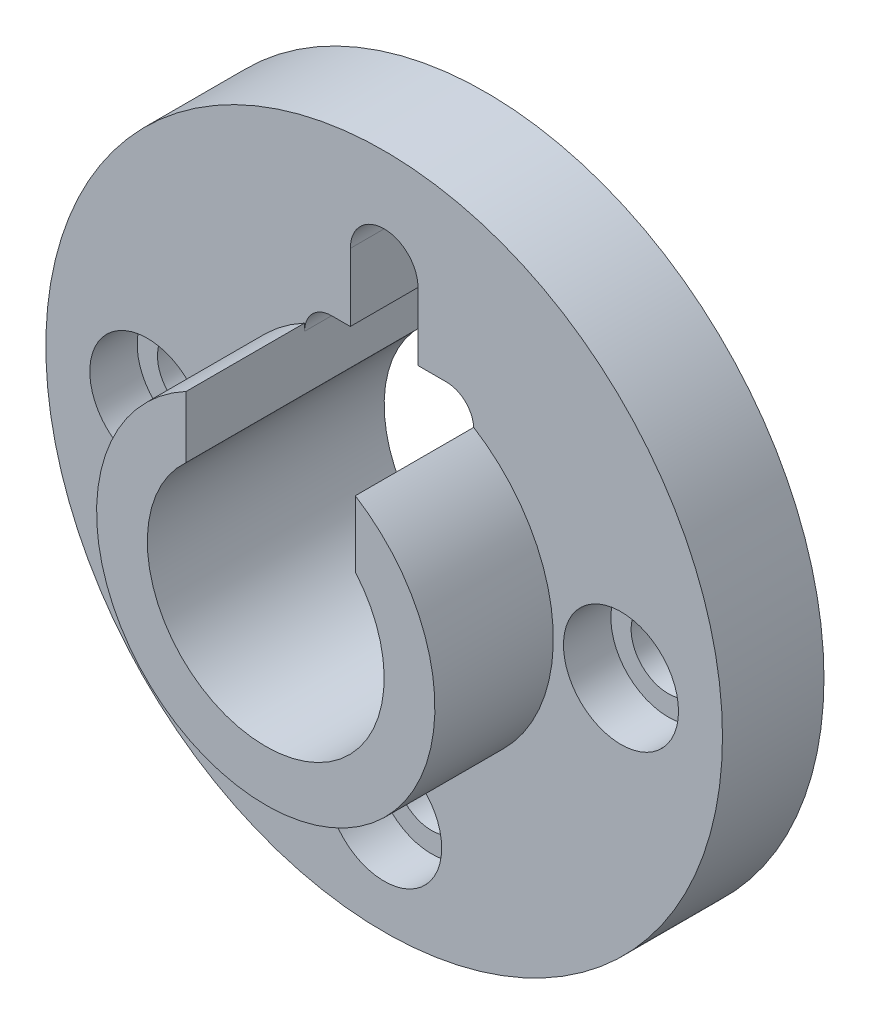
ISO-10303-21;
HEADER;
FILE_DESCRIPTION(('STEP AP214'),'2;1');
FILE_NAME('part.step','',(''),(''),'','','');
FILE_SCHEMA(('AUTOMOTIVE_DESIGN { 1 0 10303 214 1 1 1 1 }'));
ENDSEC;
DATA;
#1=APPLICATION_CONTEXT('core data for automotive mechanical design processes');
#2=APPLICATION_PROTOCOL_DEFINITION('international standard','automotive_design',2000,#1);
#3=PRODUCT_CONTEXT('',#1,'mechanical');
#4=PRODUCT('Part','Part','',(#3));
#5=PRODUCT_RELATED_PRODUCT_CATEGORY('part','',(#4));
#6=PRODUCT_DEFINITION_FORMATION('','',#4);
#7=PRODUCT_DEFINITION_CONTEXT('part definition',#1,'design');
#8=PRODUCT_DEFINITION('design','',#6,#7);
#9=PRODUCT_DEFINITION_SHAPE('','',#8);
#10=(LENGTH_UNIT() NAMED_UNIT(*) SI_UNIT(.MILLI.,.METRE.));
#11=(NAMED_UNIT(*) PLANE_ANGLE_UNIT() SI_UNIT($,.RADIAN.));
#12=(NAMED_UNIT(*) SI_UNIT($,.STERADIAN.) SOLID_ANGLE_UNIT());
#13=UNCERTAINTY_MEASURE_WITH_UNIT(LENGTH_MEASURE(1.E-05),#10,'distance_accuracy_value','');
#14=(GEOMETRIC_REPRESENTATION_CONTEXT(3) GLOBAL_UNCERTAINTY_ASSIGNED_CONTEXT((#13)) GLOBAL_UNIT_ASSIGNED_CONTEXT((#10,
#11,#12)) REPRESENTATION_CONTEXT('',''));
#15=CARTESIAN_POINT('',(0.,0.,0.));
#16=DIRECTION('',(0.,0.,1.));
#17=DIRECTION('',(1.,0.,0.));
#18=AXIS2_PLACEMENT_3D('',#15,#16,#17);
#19=CARTESIAN_POINT('',(-35.,0.,7.5));
#20=DIRECTION('',(0.,0.,-1.));
#21=DIRECTION('',(-1.,0.,0.));
#22=AXIS2_PLACEMENT_3D('',#19,#20,#21);
#23=CYLINDRICAL_SURFACE('',#22,5.5);
#24=CARTESIAN_POINT('',(-35.,0.,-7.5));
#25=DIRECTION('',(0.,0.,1.));
#26=DIRECTION('',(1.,0.,0.));
#27=AXIS2_PLACEMENT_3D('',#24,#25,#26);
#28=CIRCLE('',#27,5.5);
#29=CARTESIAN_POINT('',(-29.5,0.,-7.5));
#30=VERTEX_POINT('',#29);
#31=EDGE_CURVE('E245',#30,#30,#28,.T.);
#32=ORIENTED_EDGE('',*,*,#31,.F.);
#33=EDGE_LOOP('',(#32));
#34=FACE_BOUND('',#33,.T.);
#35=CARTESIAN_POINT('',(-35.,0.,0.5));
#36=DIRECTION('',(0.,0.,1.));
#37=DIRECTION('',(1.,0.,0.));
#38=AXIS2_PLACEMENT_3D('',#35,#36,#37);
#39=CIRCLE('',#38,5.5);
#40=CARTESIAN_POINT('',(-29.5,0.,0.5));
#41=VERTEX_POINT('',#40);
#42=EDGE_CURVE('E44',#41,#41,#39,.T.);
#43=ORIENTED_EDGE('',*,*,#42,.T.);
#44=EDGE_LOOP('',(#43));
#45=FACE_BOUND('',#44,.T.);
#46=ADVANCED_FACE('F41',(#34,#45),#23,.F.);
#47=CARTESIAN_POINT('',(35.,-2.44403693719019E-13,7.5));
#48=DIRECTION('',(0.,0.,-1.));
#49=DIRECTION('',(-1.,0.,0.));
#50=AXIS2_PLACEMENT_3D('',#47,#48,#49);
#51=CYLINDRICAL_SURFACE('',#50,5.5);
#52=CARTESIAN_POINT('',(35.,-2.44403693719019E-13,-7.5));
#53=DIRECTION('',(0.,0.,1.));
#54=DIRECTION('',(1.,0.,0.));
#55=AXIS2_PLACEMENT_3D('',#52,#53,#54);
#56=CIRCLE('',#55,5.5);
#57=CARTESIAN_POINT('',(40.5,-2.44403693719019E-13,-7.5));
#58=VERTEX_POINT('',#57);
#59=EDGE_CURVE('E242',#58,#58,#56,.T.);
#60=ORIENTED_EDGE('',*,*,#59,.F.);
#61=EDGE_LOOP('',(#60));
#62=FACE_BOUND('',#61,.T.);
#63=CARTESIAN_POINT('',(35.,-2.44403693719019E-13,0.5));
#64=DIRECTION('',(0.,0.,1.));
#65=DIRECTION('',(1.,0.,0.));
#66=AXIS2_PLACEMENT_3D('',#63,#64,#65);
#67=CIRCLE('',#66,5.5);
#68=CARTESIAN_POINT('',(40.5,-2.44403693719019E-13,0.5));
#69=VERTEX_POINT('',#68);
#70=EDGE_CURVE('E254',#69,#69,#67,.T.);
#71=ORIENTED_EDGE('',*,*,#70,.T.);
#72=EDGE_LOOP('',(#71));
#73=FACE_BOUND('',#72,.T.);
#74=ADVANCED_FACE('F351',(#62,#73),#51,.F.);
#75=CARTESIAN_POINT('',(-3.66605540578529E-13,-35.,7.5));
#76=DIRECTION('',(0.,0.,-1.));
#77=DIRECTION('',(-1.,0.,0.));
#78=AXIS2_PLACEMENT_3D('',#75,#76,#77);
#79=CYLINDRICAL_SURFACE('',#78,5.5);
#80=CARTESIAN_POINT('',(-3.66605540578529E-13,-35.,-7.5));
#81=DIRECTION('',(0.,0.,1.));
#82=DIRECTION('',(1.,0.,0.));
#83=AXIS2_PLACEMENT_3D('',#80,#81,#82);
#84=CIRCLE('',#83,5.5);
#85=CARTESIAN_POINT('',(5.49999999999963,-35.,-7.5));
#86=VERTEX_POINT('',#85);
#87=EDGE_CURVE('E239',#86,#86,#84,.T.);
#88=ORIENTED_EDGE('',*,*,#87,.F.);
#89=EDGE_LOOP('',(#88));
#90=FACE_BOUND('',#89,.T.);
#91=CARTESIAN_POINT('',(-3.66605540578529E-13,-35.,0.5));
#92=DIRECTION('',(0.,0.,1.));
#93=DIRECTION('',(1.,0.,0.));
#94=AXIS2_PLACEMENT_3D('',#91,#92,#93);
#95=CIRCLE('',#94,5.5);
#96=CARTESIAN_POINT('',(5.49999999999963,-35.,0.5));
#97=VERTEX_POINT('',#96);
#98=EDGE_CURVE('E251',#97,#97,#95,.T.);
#99=ORIENTED_EDGE('',*,*,#98,.T.);
#100=EDGE_LOOP('',(#99));
#101=FACE_BOUND('',#100,.T.);
#102=ADVANCED_FACE('F317',(#90,#101),#79,.F.);
#103=CARTESIAN_POINT('',(0.,0.,7.5));
#104=DIRECTION('',(0.,0.,1.));
#105=DIRECTION('',(1.,0.,0.));
#106=AXIS2_PLACEMENT_3D('',#103,#104,#105);
#107=PLANE('',#106);
#108=CARTESIAN_POINT('',(-35.,0.,7.5));
#109=DIRECTION('',(0.,0.,1.));
#110=DIRECTION('',(1.,0.,0.));
#111=AXIS2_PLACEMENT_3D('',#108,#109,#110);
#112=CIRCLE('',#111,8.5);
#113=CARTESIAN_POINT('',(-26.5,0.,7.5));
#114=VERTEX_POINT('',#113);
#115=EDGE_CURVE('E300',#114,#114,#112,.T.);
#116=ORIENTED_EDGE('',*,*,#115,.F.);
#117=EDGE_LOOP('',(#116));
#118=FACE_BOUND('',#117,.T.);
#119=CARTESIAN_POINT('',(35.,-2.44403693719019E-13,7.5));
#120=DIRECTION('',(0.,0.,1.));
#121=DIRECTION('',(1.,0.,0.));
#122=AXIS2_PLACEMENT_3D('',#119,#120,#121);
#123=CIRCLE('',#122,8.5);
#124=CARTESIAN_POINT('',(43.5,-2.44403693719019E-13,7.5));
#125=VERTEX_POINT('',#124);
#126=EDGE_CURVE('E297',#125,#125,#123,.T.);
#127=ORIENTED_EDGE('',*,*,#126,.F.);
#128=EDGE_LOOP('',(#127));
#129=FACE_BOUND('',#128,.T.);
#130=CARTESIAN_POINT('',(-3.66605540578529E-13,-35.,7.5));
#131=DIRECTION('',(0.,0.,1.));
#132=DIRECTION('',(1.,0.,0.));
#133=AXIS2_PLACEMENT_3D('',#130,#131,#132);
#134=CIRCLE('',#133,8.5);
#135=CARTESIAN_POINT('',(8.49999999999964,-35.,7.5));
#136=VERTEX_POINT('',#135);
#137=EDGE_CURVE('E292',#136,#136,#134,.T.);
#138=ORIENTED_EDGE('',*,*,#137,.F.);
#139=EDGE_LOOP('',(#138));
#140=FACE_BOUND('',#139,.T.);
#141=CARTESIAN_POINT('',(0.,0.,7.5));
#142=DIRECTION('',(0.,0.,1.));
#143=DIRECTION('',(1.,0.,0.));
#144=AXIS2_PLACEMENT_3D('',#141,#142,#143);
#145=CIRCLE('',#144,50.);
#146=CARTESIAN_POINT('',(50.,0.,7.5));
#147=VERTEX_POINT('',#146);
#148=EDGE_CURVE('E49',#147,#147,#145,.T.);
#149=ORIENTED_EDGE('',*,*,#148,.T.);
#150=EDGE_LOOP('',(#149));
#151=FACE_BOUND('',#150,.T.);
#152=CARTESIAN_POINT('',(9.23698245276787,21.,7.5));
#153=DIRECTION('',(0.,0.,1.));
#154=DIRECTION('',(-1.,0.,0.));
#155=AXIS2_PLACEMENT_3D('',#152,#153,#154);
#156=CIRCLE('',#155,4.);
#157=CARTESIAN_POINT('',(13.2369824527679,21.,7.5));
#158=VERTEX_POINT('',#157);
#159=CARTESIAN_POINT('',(9.23698245276784,25.,7.5));
#160=VERTEX_POINT('',#159);
#161=EDGE_CURVE('E194',#158,#160,#156,.T.);
#162=ORIENTED_EDGE('',*,*,#161,.F.);
#163=DIRECTION('',(0.,1.,0.));
#164=VECTOR('',#163,1.);
#165=CARTESIAN_POINT('',(13.2369824527679,0.,7.5));
#166=LINE('',#165,#164);
#167=CARTESIAN_POINT('',(13.2369824527679,21.2080714716147,7.5));
#168=VERTEX_POINT('',#167);
#169=EDGE_CURVE('E171',#158,#168,#166,.T.);
#170=ORIENTED_EDGE('',*,*,#169,.T.);
#171=CARTESIAN_POINT('',(0.,0.,7.5));
#172=DIRECTION('',(0.,0.,1.));
#173=DIRECTION('',(1.,0.,0.));
#174=AXIS2_PLACEMENT_3D('',#171,#172,#173);
#175=CIRCLE('',#174,25.);
#176=CARTESIAN_POINT('',(-11.7630175472321,22.059723891824,7.5));
#177=VERTEX_POINT('',#176);
#178=EDGE_CURVE('E170',#168,#177,#175,.F.);
#179=ORIENTED_EDGE('',*,*,#178,.T.);
#180=DIRECTION('',(0.,-1.,0.));
#181=VECTOR('',#180,1.);
#182=CARTESIAN_POINT('',(-11.7630175472321,0.,7.5));
#183=LINE('',#182,#181);
#184=CARTESIAN_POINT('',(-11.7630175472321,21.,7.5));
#185=VERTEX_POINT('',#184);
#186=EDGE_CURVE('E176',#177,#185,#183,.T.);
#187=ORIENTED_EDGE('',*,*,#186,.T.);
#188=CARTESIAN_POINT('',(-7.76301754723214,21.,7.5));
#189=DIRECTION('',(0.,0.,1.));
#190=DIRECTION('',(1.,0.,0.));
#191=AXIS2_PLACEMENT_3D('',#188,#189,#190);
#192=CIRCLE('',#191,4.);
#193=CARTESIAN_POINT('',(-7.76301754723211,25.,7.5));
#194=VERTEX_POINT('',#193);
#195=EDGE_CURVE('E190',#194,#185,#192,.T.);
#196=ORIENTED_EDGE('',*,*,#195,.F.);
#197=DIRECTION('',(-1.,0.,0.));
#198=VECTOR('',#197,1.);
#199=CARTESIAN_POINT('',(-7.76301754723211,25.,7.5));
#200=LINE('',#199,#198);
#201=CARTESIAN_POINT('',(-5.,25.,7.5));
#202=VERTEX_POINT('',#201);
#203=EDGE_CURVE('E189',#202,#194,#200,.T.);
#204=ORIENTED_EDGE('',*,*,#203,.F.);
#205=DIRECTION('',(0.,-1.,0.));
#206=VECTOR('',#205,1.);
#207=CARTESIAN_POINT('',(-5.,35.,7.5));
#208=LINE('',#207,#206);
#209=CARTESIAN_POINT('',(-5.,35.,7.5));
#210=VERTEX_POINT('',#209);
#211=EDGE_CURVE('E183',#210,#202,#208,.T.);
#212=ORIENTED_EDGE('',*,*,#211,.F.);
#213=CARTESIAN_POINT('',(0.,35.,7.5));
#214=DIRECTION('',(0.,0.,1.));
#215=DIRECTION('',(1.,0.,0.));
#216=AXIS2_PLACEMENT_3D('',#213,#214,#215);
#217=CIRCLE('',#216,5.);
#218=CARTESIAN_POINT('',(5.,35.,7.5));
#219=VERTEX_POINT('',#218);
#220=EDGE_CURVE('E181',#219,#210,#217,.T.);
#221=ORIENTED_EDGE('',*,*,#220,.F.);
#222=DIRECTION('',(0.,1.,0.));
#223=VECTOR('',#222,1.);
#224=CARTESIAN_POINT('',(5.,35.,7.5));
#225=LINE('',#224,#223);
#226=CARTESIAN_POINT('',(5.,25.,7.5));
#227=VERTEX_POINT('',#226);
#228=EDGE_CURVE('E196',#227,#219,#225,.T.);
#229=ORIENTED_EDGE('',*,*,#228,.F.);
#230=DIRECTION('',(-1.,0.,0.));
#231=VECTOR('',#230,1.);
#232=CARTESIAN_POINT('',(5.,25.,7.5));
#233=LINE('',#232,#231);
#234=EDGE_CURVE('E193',#160,#227,#233,.T.);
#235=ORIENTED_EDGE('',*,*,#234,.F.);
#236=EDGE_LOOP('',(#162,#170,#179,#187,#196,#204,#212,#221,#229,#235));
#237=FACE_BOUND('',#236,.T.);
#238=ADVANCED_FACE('F312',(#118,#129,#140,#151,#237),#107,.T.);
#239=CARTESIAN_POINT('',(0.,0.,-7.5));
#240=DIRECTION('',(0.,0.,1.));
#241=DIRECTION('',(1.,0.,0.));
#242=AXIS2_PLACEMENT_3D('',#239,#240,#241);
#243=PLANE('',#242);
#244=CARTESIAN_POINT('',(0.,0.,-7.5));
#245=DIRECTION('',(0.,0.,1.));
#246=DIRECTION('',(1.,0.,0.));
#247=AXIS2_PLACEMENT_3D('',#244,#245,#246);
#248=CIRCLE('',#247,50.);
#249=CARTESIAN_POINT('',(50.,0.,-7.5));
#250=VERTEX_POINT('',#249);
#251=EDGE_CURVE('E249',#250,#250,#248,.T.);
#252=ORIENTED_EDGE('',*,*,#251,.F.);
#253=EDGE_LOOP('',(#252));
#254=FACE_BOUND('',#253,.T.);
#255=ORIENTED_EDGE('',*,*,#31,.T.);
#256=EDGE_LOOP('',(#255));
#257=FACE_BOUND('',#256,.T.);
#258=ORIENTED_EDGE('',*,*,#59,.T.);
#259=EDGE_LOOP('',(#258));
#260=FACE_BOUND('',#259,.T.);
#261=ORIENTED_EDGE('',*,*,#87,.T.);
#262=EDGE_LOOP('',(#261));
#263=FACE_BOUND('',#262,.T.);
#264=DIRECTION('',(0.,1.,0.));
#265=VECTOR('',#264,1.);
#266=CARTESIAN_POINT('',(13.2369824527679,0.,-7.5));
#267=LINE('',#266,#265);
#268=CARTESIAN_POINT('',(13.2369824527679,21.,-7.5));
#269=VERTEX_POINT('',#268);
#270=CARTESIAN_POINT('',(13.2369824527679,21.2080714716147,-7.5));
#271=VERTEX_POINT('',#270);
#272=EDGE_CURVE('E169',#269,#271,#267,.T.);
#273=ORIENTED_EDGE('',*,*,#272,.F.);
#274=CARTESIAN_POINT('',(9.23698245276787,21.,-7.5));
#275=DIRECTION('',(0.,0.,1.));
#276=DIRECTION('',(-1.,0.,0.));
#277=AXIS2_PLACEMENT_3D('',#274,#275,#276);
#278=CIRCLE('',#277,4.);
#279=CARTESIAN_POINT('',(9.23698245276784,25.,-7.5));
#280=VERTEX_POINT('',#279);
#281=EDGE_CURVE('E211',#269,#280,#278,.T.);
#282=ORIENTED_EDGE('',*,*,#281,.T.);
#283=DIRECTION('',(-1.,0.,0.));
#284=VECTOR('',#283,1.);
#285=CARTESIAN_POINT('',(5.,25.,-7.5));
#286=LINE('',#285,#284);
#287=CARTESIAN_POINT('',(5.,25.,-7.5));
#288=VERTEX_POINT('',#287);
#289=EDGE_CURVE('E212',#280,#288,#286,.T.);
#290=ORIENTED_EDGE('',*,*,#289,.T.);
#291=DIRECTION('',(0.,1.,0.));
#292=VECTOR('',#291,1.);
#293=CARTESIAN_POINT('',(5.,35.,-7.5));
#294=LINE('',#293,#292);
#295=CARTESIAN_POINT('',(5.,35.,-7.5));
#296=VERTEX_POINT('',#295);
#297=EDGE_CURVE('E186',#288,#296,#294,.T.);
#298=ORIENTED_EDGE('',*,*,#297,.T.);
#299=CARTESIAN_POINT('',(0.,35.,-7.5));
#300=DIRECTION('',(0.,0.,1.));
#301=DIRECTION('',(1.,0.,0.));
#302=AXIS2_PLACEMENT_3D('',#299,#300,#301);
#303=CIRCLE('',#302,5.);
#304=CARTESIAN_POINT('',(-5.,35.,-7.5));
#305=VERTEX_POINT('',#304);
#306=EDGE_CURVE('E185',#296,#305,#303,.T.);
#307=ORIENTED_EDGE('',*,*,#306,.T.);
#308=DIRECTION('',(0.,-1.,0.));
#309=VECTOR('',#308,1.);
#310=CARTESIAN_POINT('',(-5.,35.,-7.5));
#311=LINE('',#310,#309);
#312=CARTESIAN_POINT('',(-5.,25.,-7.5));
#313=VERTEX_POINT('',#312);
#314=EDGE_CURVE('E201',#305,#313,#311,.T.);
#315=ORIENTED_EDGE('',*,*,#314,.T.);
#316=DIRECTION('',(-1.,0.,0.));
#317=VECTOR('',#316,1.);
#318=CARTESIAN_POINT('',(-7.76301754723211,25.,-7.5));
#319=LINE('',#318,#317);
#320=CARTESIAN_POINT('',(-7.76301754723211,25.,-7.5));
#321=VERTEX_POINT('',#320);
#322=EDGE_CURVE('E206',#313,#321,#319,.T.);
#323=ORIENTED_EDGE('',*,*,#322,.T.);
#324=CARTESIAN_POINT('',(-7.76301754723214,21.,-7.5));
#325=DIRECTION('',(0.,0.,1.));
#326=DIRECTION('',(1.,0.,0.));
#327=AXIS2_PLACEMENT_3D('',#324,#325,#326);
#328=CIRCLE('',#327,4.);
#329=CARTESIAN_POINT('',(-11.7630175472321,21.,-7.5));
#330=VERTEX_POINT('',#329);
#331=EDGE_CURVE('E207',#321,#330,#328,.T.);
#332=ORIENTED_EDGE('',*,*,#331,.T.);
#333=DIRECTION('',(0.,-1.,0.));
#334=VECTOR('',#333,1.);
#335=CARTESIAN_POINT('',(-11.7630175472321,0.,-7.5));
#336=LINE('',#335,#334);
#337=CARTESIAN_POINT('',(-11.7630175472321,22.059723891824,-7.5));
#338=VERTEX_POINT('',#337);
#339=EDGE_CURVE('E61',#338,#330,#336,.T.);
#340=ORIENTED_EDGE('',*,*,#339,.F.);
#341=CARTESIAN_POINT('',(0.,0.,-7.5));
#342=DIRECTION('',(0.,0.,1.));
#343=DIRECTION('',(1.,0.,0.));
#344=AXIS2_PLACEMENT_3D('',#341,#342,#343);
#345=CIRCLE('',#344,25.);
#346=EDGE_CURVE('E11',#271,#338,#345,.F.);
#347=ORIENTED_EDGE('',*,*,#346,.F.);
#348=EDGE_LOOP('',(#273,#282,#290,#298,#307,#315,#323,#332,#340,#347));
#349=FACE_BOUND('',#348,.T.);
#350=ADVANCED_FACE('F318',(#254,#257,#260,#263,#349),#243,.F.);
#351=CARTESIAN_POINT('',(0.,0.,7.5));
#352=DIRECTION('',(0.,0.,-1.));
#353=DIRECTION('',(-1.,0.,0.));
#354=AXIS2_PLACEMENT_3D('',#351,#352,#353);
#355=CYLINDRICAL_SURFACE('',#354,50.);
#356=ORIENTED_EDGE('',*,*,#148,.F.);
#357=EDGE_LOOP('',(#356));
#358=FACE_BOUND('',#357,.T.);
#359=ORIENTED_EDGE('',*,*,#251,.T.);
#360=EDGE_LOOP('',(#359));
#361=FACE_BOUND('',#360,.T.);
#362=ADVANCED_FACE('F43',(#358,#361),#355,.T.);
#363=CARTESIAN_POINT('',(0.,35.,7.5));
#364=DIRECTION('',(0.,0.,-1.));
#365=DIRECTION('',(-1.,0.,0.));
#366=AXIS2_PLACEMENT_3D('',#363,#364,#365);
#367=CYLINDRICAL_SURFACE('',#366,5.);
#368=ORIENTED_EDGE('',*,*,#306,.F.);
#369=DIRECTION('',(0.,0.,-1.));
#370=VECTOR('',#369,1.);
#371=CARTESIAN_POINT('',(5.,35.,7.5));
#372=LINE('',#371,#370);
#373=EDGE_CURVE('E199',#219,#296,#372,.T.);
#374=ORIENTED_EDGE('',*,*,#373,.F.);
#375=ORIENTED_EDGE('',*,*,#220,.T.);
#376=DIRECTION('',(0.,0.,-1.));
#377=VECTOR('',#376,1.);
#378=CARTESIAN_POINT('',(-5.,35.,7.5));
#379=LINE('',#378,#377);
#380=EDGE_CURVE('E237',#210,#305,#379,.T.);
#381=ORIENTED_EDGE('',*,*,#380,.T.);
#382=EDGE_LOOP('',(#368,#374,#375,#381));
#383=FACE_BOUND('',#382,.T.);
#384=ADVANCED_FACE('F347',(#383),#367,.F.);
#385=CARTESIAN_POINT('',(-5.,35.,7.5));
#386=DIRECTION('',(1.,0.,0.));
#387=DIRECTION('',(0.,1.,0.));
#388=AXIS2_PLACEMENT_3D('',#385,#386,#387);
#389=PLANE('',#388);
#390=ORIENTED_EDGE('',*,*,#314,.F.);
#391=ORIENTED_EDGE('',*,*,#380,.F.);
#392=ORIENTED_EDGE('',*,*,#211,.T.);
#393=DIRECTION('',(0.,0.,-1.));
#394=VECTOR('',#393,1.);
#395=CARTESIAN_POINT('',(-5.,25.,7.5));
#396=LINE('',#395,#394);
#397=EDGE_CURVE('E231',#202,#313,#396,.T.);
#398=ORIENTED_EDGE('',*,*,#397,.T.);
#399=EDGE_LOOP('',(#390,#391,#392,#398));
#400=FACE_BOUND('',#399,.T.);
#401=ADVANCED_FACE('F370',(#400),#389,.T.);
#402=CARTESIAN_POINT('',(-7.76301754723211,25.,7.5));
#403=DIRECTION('',(0.,-1.,0.));
#404=DIRECTION('',(0.,0.,-1.));
#405=AXIS2_PLACEMENT_3D('',#402,#403,#404);
#406=PLANE('',#405);
#407=ORIENTED_EDGE('',*,*,#322,.F.);
#408=ORIENTED_EDGE('',*,*,#397,.F.);
#409=ORIENTED_EDGE('',*,*,#203,.T.);
#410=DIRECTION('',(0.,0.,-1.));
#411=VECTOR('',#410,1.);
#412=CARTESIAN_POINT('',(-7.76301754723211,25.,7.5));
#413=LINE('',#412,#411);
#414=EDGE_CURVE('E235',#194,#321,#413,.T.);
#415=ORIENTED_EDGE('',*,*,#414,.T.);
#416=EDGE_LOOP('',(#407,#408,#409,#415));
#417=FACE_BOUND('',#416,.T.);
#418=ADVANCED_FACE('F371',(#417),#406,.T.);
#419=CARTESIAN_POINT('',(-7.76301754723214,21.,7.5));
#420=DIRECTION('',(0.,0.,-1.));
#421=DIRECTION('',(-1.,0.,0.));
#422=AXIS2_PLACEMENT_3D('',#419,#420,#421);
#423=CYLINDRICAL_SURFACE('',#422,4.);
#424=ORIENTED_EDGE('',*,*,#331,.F.);
#425=ORIENTED_EDGE('',*,*,#414,.F.);
#426=ORIENTED_EDGE('',*,*,#195,.T.);
#427=DIRECTION('',(0.,0.,-1.));
#428=VECTOR('',#427,1.);
#429=CARTESIAN_POINT('',(-11.7630175472321,21.,7.5));
#430=LINE('',#429,#428);
#431=EDGE_CURVE('E230',#185,#330,#430,.T.);
#432=ORIENTED_EDGE('',*,*,#431,.T.);
#433=EDGE_LOOP('',(#424,#425,#426,#432));
#434=FACE_BOUND('',#433,.T.);
#435=ADVANCED_FACE('F374',(#434),#423,.F.);
#436=CARTESIAN_POINT('',(-11.7630175472321,12.9569061964463,7.5));
#437=DIRECTION('',(1.,0.,0.));
#438=DIRECTION('',(0.,0.,-1.));
#439=AXIS2_PLACEMENT_3D('',#436,#437,#438);
#440=PLANE('',#439);
#441=DIRECTION('',(0.,0.,-1.));
#442=VECTOR('',#441,1.);
#443=CARTESIAN_POINT('',(-11.7630175472321,12.9569061964463,7.5));
#444=LINE('',#443,#442);
#445=CARTESIAN_POINT('',(-11.7630175472321,12.9569061964463,25.));
#446=VERTEX_POINT('',#445);
#447=CARTESIAN_POINT('',(-11.7630175472321,12.9569061964463,-10.));
#448=VERTEX_POINT('',#447);
#449=EDGE_CURVE('E229',#446,#448,#444,.T.);
#450=ORIENTED_EDGE('',*,*,#449,.T.);
#451=DIRECTION('',(0.,1.,0.));
#452=VECTOR('',#451,1.);
#453=CARTESIAN_POINT('',(-11.7630175472321,12.9569061964463,-10.));
#454=LINE('',#453,#452);
#455=CARTESIAN_POINT('',(-11.7630175472321,22.059723891824,-10.));
#456=VERTEX_POINT('',#455);
#457=EDGE_CURVE('E162',#448,#456,#454,.T.);
#458=ORIENTED_EDGE('',*,*,#457,.T.);
#459=DIRECTION('',(0.,0.,-1.));
#460=VECTOR('',#459,1.);
#461=CARTESIAN_POINT('',(-11.7630175472321,22.059723891824,25.));
#462=LINE('',#461,#460);
#463=EDGE_CURVE('E281',#338,#456,#462,.T.);
#464=ORIENTED_EDGE('',*,*,#463,.F.);
#465=ORIENTED_EDGE('',*,*,#339,.T.);
#466=ORIENTED_EDGE('',*,*,#431,.F.);
#467=ORIENTED_EDGE('',*,*,#186,.F.);
#468=CARTESIAN_POINT('',(-11.7630175472321,22.059723891824,25.));
#469=VERTEX_POINT('',#468);
#470=EDGE_CURVE('E174',#469,#177,#462,.T.);
#471=ORIENTED_EDGE('',*,*,#470,.F.);
#472=DIRECTION('',(0.,1.,0.));
#473=VECTOR('',#472,1.);
#474=CARTESIAN_POINT('',(-11.7630175472321,12.9569061964463,25.));
#475=LINE('',#474,#473);
#476=EDGE_CURVE('E157',#446,#469,#475,.T.);
#477=ORIENTED_EDGE('',*,*,#476,.F.);
#478=EDGE_LOOP('',(#450,#458,#464,#465,#466,#467,#471,#477));
#479=FACE_BOUND('',#478,.T.);
#480=ADVANCED_FACE('F278',(#479),#440,.T.);
#481=CARTESIAN_POINT('',(0.,0.,7.5));
#482=DIRECTION('',(0.,0.,-1.));
#483=DIRECTION('',(-1.,0.,0.));
#484=AXIS2_PLACEMENT_3D('',#481,#482,#483);
#485=CYLINDRICAL_SURFACE('',#484,17.5);
#486=DIRECTION('',(0.,0.,-1.));
#487=VECTOR('',#486,1.);
#488=CARTESIAN_POINT('',(13.2369824527679,11.4469338927556,7.5));
#489=LINE('',#488,#487);
#490=CARTESIAN_POINT('',(13.2369824527679,11.4469338927555,25.));
#491=VERTEX_POINT('',#490);
#492=CARTESIAN_POINT('',(13.2369824527679,11.4469338927555,-10.));
#493=VERTEX_POINT('',#492);
#494=EDGE_CURVE('E149',#491,#493,#489,.T.);
#495=ORIENTED_EDGE('',*,*,#494,.T.);
#496=CARTESIAN_POINT('',(0.,0.,-10.));
#497=DIRECTION('',(0.,0.,-1.));
#498=DIRECTION('',(1.,0.,0.));
#499=AXIS2_PLACEMENT_3D('',#496,#497,#498);
#500=CIRCLE('',#499,17.5);
#501=EDGE_CURVE('E269',#493,#448,#500,.T.);
#502=ORIENTED_EDGE('',*,*,#501,.T.);
#503=ORIENTED_EDGE('',*,*,#449,.F.);
#504=CARTESIAN_POINT('',(0.,0.,25.));
#505=DIRECTION('',(0.,0.,-1.));
#506=DIRECTION('',(1.,0.,0.));
#507=AXIS2_PLACEMENT_3D('',#504,#505,#506);
#508=CIRCLE('',#507,17.5);
#509=EDGE_CURVE('E153',#491,#446,#508,.T.);
#510=ORIENTED_EDGE('',*,*,#509,.F.);
#511=EDGE_LOOP('',(#495,#502,#503,#510));
#512=FACE_BOUND('',#511,.T.);
#513=ADVANCED_FACE('F381',(#512),#485,.F.);
#514=CARTESIAN_POINT('',(13.2369824527679,11.4469338927556,7.5));
#515=DIRECTION('',(-1.,0.,0.));
#516=DIRECTION('',(0.,0.,1.));
#517=AXIS2_PLACEMENT_3D('',#514,#515,#516);
#518=PLANE('',#517);
#519=DIRECTION('',(0.,0.,-1.));
#520=VECTOR('',#519,1.);
#521=CARTESIAN_POINT('',(13.2369824527679,21.,7.5));
#522=LINE('',#521,#520);
#523=EDGE_CURVE('E223',#158,#269,#522,.T.);
#524=ORIENTED_EDGE('',*,*,#523,.T.);
#525=ORIENTED_EDGE('',*,*,#272,.T.);
#526=DIRECTION('',(0.,0.,-1.));
#527=VECTOR('',#526,1.);
#528=CARTESIAN_POINT('',(13.2369824527679,21.2080714716147,25.));
#529=LINE('',#528,#527);
#530=CARTESIAN_POINT('',(13.2369824527679,21.2080714716147,-10.));
#531=VERTEX_POINT('',#530);
#532=EDGE_CURVE('E166',#271,#531,#529,.T.);
#533=ORIENTED_EDGE('',*,*,#532,.T.);
#534=DIRECTION('',(0.,-1.,0.));
#535=VECTOR('',#534,1.);
#536=CARTESIAN_POINT('',(13.2369824527679,11.4469338927556,-10.));
#537=LINE('',#536,#535);
#538=EDGE_CURVE('E264',#531,#493,#537,.T.);
#539=ORIENTED_EDGE('',*,*,#538,.T.);
#540=ORIENTED_EDGE('',*,*,#494,.F.);
#541=DIRECTION('',(0.,-1.,0.));
#542=VECTOR('',#541,1.);
#543=CARTESIAN_POINT('',(13.2369824527679,11.4469338927556,25.));
#544=LINE('',#543,#542);
#545=CARTESIAN_POINT('',(13.2369824527679,21.2080714716147,25.));
#546=VERTEX_POINT('',#545);
#547=EDGE_CURVE('E143',#546,#491,#544,.T.);
#548=ORIENTED_EDGE('',*,*,#547,.F.);
#549=EDGE_CURVE('E148',#546,#168,#529,.T.);
#550=ORIENTED_EDGE('',*,*,#549,.T.);
#551=ORIENTED_EDGE('',*,*,#169,.F.);
#552=EDGE_LOOP('',(#524,#525,#533,#539,#540,#548,#550,#551));
#553=FACE_BOUND('',#552,.T.);
#554=ADVANCED_FACE('F145',(#553),#518,.T.);
#555=CARTESIAN_POINT('',(9.23698245276787,21.,7.5));
#556=DIRECTION('',(0.,0.,-1.));
#557=DIRECTION('',(-1.,0.,0.));
#558=AXIS2_PLACEMENT_3D('',#555,#556,#557);
#559=CYLINDRICAL_SURFACE('',#558,4.);
#560=ORIENTED_EDGE('',*,*,#281,.F.);
#561=ORIENTED_EDGE('',*,*,#523,.F.);
#562=ORIENTED_EDGE('',*,*,#161,.T.);
#563=DIRECTION('',(0.,0.,-1.));
#564=VECTOR('',#563,1.);
#565=CARTESIAN_POINT('',(9.23698245276784,25.,7.5));
#566=LINE('',#565,#564);
#567=EDGE_CURVE('E224',#160,#280,#566,.T.);
#568=ORIENTED_EDGE('',*,*,#567,.T.);
#569=EDGE_LOOP('',(#560,#561,#562,#568));
#570=FACE_BOUND('',#569,.T.);
#571=ADVANCED_FACE('F331',(#570),#559,.F.);
#572=CARTESIAN_POINT('',(5.,25.,7.5));
#573=DIRECTION('',(0.,-1.,0.));
#574=DIRECTION('',(0.,0.,-1.));
#575=AXIS2_PLACEMENT_3D('',#572,#573,#574);
#576=PLANE('',#575);
#577=ORIENTED_EDGE('',*,*,#289,.F.);
#578=ORIENTED_EDGE('',*,*,#567,.F.);
#579=ORIENTED_EDGE('',*,*,#234,.T.);
#580=DIRECTION('',(0.,0.,-1.));
#581=VECTOR('',#580,1.);
#582=CARTESIAN_POINT('',(5.,25.,7.5));
#583=LINE('',#582,#581);
#584=EDGE_CURVE('E222',#227,#288,#583,.T.);
#585=ORIENTED_EDGE('',*,*,#584,.T.);
#586=EDGE_LOOP('',(#577,#578,#579,#585));
#587=FACE_BOUND('',#586,.T.);
#588=ADVANCED_FACE('F337',(#587),#576,.T.);
#589=CARTESIAN_POINT('',(5.,35.,7.5));
#590=DIRECTION('',(-1.,0.,0.));
#591=DIRECTION('',(0.,-1.,0.));
#592=AXIS2_PLACEMENT_3D('',#589,#590,#591);
#593=PLANE('',#592);
#594=ORIENTED_EDGE('',*,*,#297,.F.);
#595=ORIENTED_EDGE('',*,*,#584,.F.);
#596=ORIENTED_EDGE('',*,*,#228,.T.);
#597=ORIENTED_EDGE('',*,*,#373,.T.);
#598=EDGE_LOOP('',(#594,#595,#596,#597));
#599=FACE_BOUND('',#598,.T.);
#600=ADVANCED_FACE('F391',(#599),#593,.T.);
#601=CARTESIAN_POINT('',(0.,0.,-10.));
#602=DIRECTION('',(0.,0.,1.));
#603=DIRECTION('',(1.,0.,0.));
#604=AXIS2_PLACEMENT_3D('',#601,#602,#603);
#605=PLANE('',#604);
#606=CARTESIAN_POINT('',(0.,0.,-10.));
#607=DIRECTION('',(0.,0.,1.));
#608=DIRECTION('',(1.,0.,0.));
#609=AXIS2_PLACEMENT_3D('',#606,#607,#608);
#610=CIRCLE('',#609,25.);
#611=EDGE_CURVE('E261',#456,#531,#610,.T.);
#612=ORIENTED_EDGE('',*,*,#611,.F.);
#613=ORIENTED_EDGE('',*,*,#457,.F.);
#614=ORIENTED_EDGE('',*,*,#501,.F.);
#615=ORIENTED_EDGE('',*,*,#538,.F.);
#616=EDGE_LOOP('',(#612,#613,#614,#615));
#617=FACE_BOUND('',#616,.T.);
#618=ADVANCED_FACE('F285',(#617),#605,.F.);
#619=CARTESIAN_POINT('',(0.,0.,25.));
#620=DIRECTION('',(0.,0.,-1.));
#621=DIRECTION('',(-1.,0.,0.));
#622=AXIS2_PLACEMENT_3D('',#619,#620,#621);
#623=CYLINDRICAL_SURFACE('',#622,25.);
#624=ORIENTED_EDGE('',*,*,#532,.F.);
#625=ORIENTED_EDGE('',*,*,#346,.T.);
#626=ORIENTED_EDGE('',*,*,#463,.T.);
#627=ORIENTED_EDGE('',*,*,#611,.T.);
#628=EDGE_LOOP('',(#624,#625,#626,#627));
#629=FACE_BOUND('',#628,.T.);
#630=ADVANCED_FACE('F287',(#629),#623,.T.);
#631=ORIENTED_EDGE('',*,*,#178,.F.);
#632=ORIENTED_EDGE('',*,*,#549,.F.);
#633=CARTESIAN_POINT('',(0.,0.,25.));
#634=DIRECTION('',(0.,0.,1.));
#635=DIRECTION('',(1.,0.,0.));
#636=AXIS2_PLACEMENT_3D('',#633,#634,#635);
#637=CIRCLE('',#636,25.);
#638=EDGE_CURVE('E152',#469,#546,#637,.T.);
#639=ORIENTED_EDGE('',*,*,#638,.F.);
#640=ORIENTED_EDGE('',*,*,#470,.T.);
#641=EDGE_LOOP('',(#631,#632,#639,#640));
#642=FACE_BOUND('',#641,.T.);
#643=ADVANCED_FACE('F164',(#642),#623,.T.);
#644=CARTESIAN_POINT('',(0.,0.,25.));
#645=DIRECTION('',(0.,0.,1.));
#646=DIRECTION('',(1.,0.,0.));
#647=AXIS2_PLACEMENT_3D('',#644,#645,#646);
#648=PLANE('',#647);
#649=ORIENTED_EDGE('',*,*,#638,.T.);
#650=ORIENTED_EDGE('',*,*,#547,.T.);
#651=ORIENTED_EDGE('',*,*,#509,.T.);
#652=ORIENTED_EDGE('',*,*,#476,.T.);
#653=EDGE_LOOP('',(#649,#650,#651,#652));
#654=FACE_BOUND('',#653,.T.);
#655=ADVANCED_FACE('F160',(#654),#648,.T.);
#656=CARTESIAN_POINT('',(-3.66605540578529E-13,-35.,0.5));
#657=DIRECTION('',(0.,0.,1.));
#658=DIRECTION('',(1.,0.,0.));
#659=AXIS2_PLACEMENT_3D('',#656,#657,#658);
#660=CYLINDRICAL_SURFACE('',#659,8.5);
#661=CARTESIAN_POINT('',(-3.66605540578529E-13,-35.,0.5));
#662=DIRECTION('',(0.,0.,1.));
#663=DIRECTION('',(1.,0.,0.));
#664=AXIS2_PLACEMENT_3D('',#661,#662,#663);
#665=CIRCLE('',#664,8.5);
#666=CARTESIAN_POINT('',(8.49999999999964,-35.,0.5));
#667=VERTEX_POINT('',#666);
#668=EDGE_CURVE('E289',#667,#667,#665,.T.);
#669=ORIENTED_EDGE('',*,*,#668,.F.);
#670=EDGE_LOOP('',(#669));
#671=FACE_BOUND('',#670,.T.);
#672=ORIENTED_EDGE('',*,*,#137,.T.);
#673=EDGE_LOOP('',(#672));
#674=FACE_BOUND('',#673,.T.);
#675=ADVANCED_FACE('F396',(#671,#674),#660,.F.);
#676=CARTESIAN_POINT('',(-3.66605540578529E-13,-35.,0.5));
#677=DIRECTION('',(0.,0.,1.));
#678=DIRECTION('',(1.,0.,0.));
#679=AXIS2_PLACEMENT_3D('',#676,#677,#678);
#680=PLANE('',#679);
#681=ORIENTED_EDGE('',*,*,#98,.F.);
#682=EDGE_LOOP('',(#681));
#683=FACE_BOUND('',#682,.T.);
#684=ORIENTED_EDGE('',*,*,#668,.T.);
#685=EDGE_LOOP('',(#684));
#686=FACE_BOUND('',#685,.T.);
#687=ADVANCED_FACE('F398',(#683,#686),#680,.T.);
#688=CARTESIAN_POINT('',(35.,-2.44403693719019E-13,0.5));
#689=DIRECTION('',(0.,0.,1.));
#690=DIRECTION('',(1.,0.,0.));
#691=AXIS2_PLACEMENT_3D('',#688,#689,#690);
#692=CYLINDRICAL_SURFACE('',#691,8.5);
#693=CARTESIAN_POINT('',(35.,-2.44403693719019E-13,0.5));
#694=DIRECTION('',(0.,0.,1.));
#695=DIRECTION('',(1.,0.,0.));
#696=AXIS2_PLACEMENT_3D('',#693,#694,#695);
#697=CIRCLE('',#696,8.5);
#698=CARTESIAN_POINT('',(43.5,-2.44403693719019E-13,0.5));
#699=VERTEX_POINT('',#698);
#700=EDGE_CURVE('E294',#699,#699,#697,.T.);
#701=ORIENTED_EDGE('',*,*,#700,.F.);
#702=EDGE_LOOP('',(#701));
#703=FACE_BOUND('',#702,.T.);
#704=ORIENTED_EDGE('',*,*,#126,.T.);
#705=EDGE_LOOP('',(#704));
#706=FACE_BOUND('',#705,.T.);
#707=ADVANCED_FACE('F401',(#703,#706),#692,.F.);
#708=CARTESIAN_POINT('',(35.,-2.44403693719019E-13,0.5));
#709=DIRECTION('',(0.,0.,1.));
#710=DIRECTION('',(1.,0.,0.));
#711=AXIS2_PLACEMENT_3D('',#708,#709,#710);
#712=PLANE('',#711);
#713=ORIENTED_EDGE('',*,*,#70,.F.);
#714=EDGE_LOOP('',(#713));
#715=FACE_BOUND('',#714,.T.);
#716=ORIENTED_EDGE('',*,*,#700,.T.);
#717=EDGE_LOOP('',(#716));
#718=FACE_BOUND('',#717,.T.);
#719=ADVANCED_FACE('F313',(#715,#718),#712,.T.);
#720=CARTESIAN_POINT('',(-35.,0.,0.5));
#721=DIRECTION('',(0.,0.,1.));
#722=DIRECTION('',(1.,0.,0.));
#723=AXIS2_PLACEMENT_3D('',#720,#721,#722);
#724=CYLINDRICAL_SURFACE('',#723,8.5);
#725=CARTESIAN_POINT('',(-35.,0.,0.5));
#726=DIRECTION('',(0.,0.,1.));
#727=DIRECTION('',(1.,0.,0.));
#728=AXIS2_PLACEMENT_3D('',#725,#726,#727);
#729=CIRCLE('',#728,8.5);
#730=CARTESIAN_POINT('',(-26.5,0.,0.5));
#731=VERTEX_POINT('',#730);
#732=EDGE_CURVE('E258',#731,#731,#729,.T.);
#733=ORIENTED_EDGE('',*,*,#732,.F.);
#734=EDGE_LOOP('',(#733));
#735=FACE_BOUND('',#734,.T.);
#736=ORIENTED_EDGE('',*,*,#115,.T.);
#737=EDGE_LOOP('',(#736));
#738=FACE_BOUND('',#737,.T.);
#739=ADVANCED_FACE('F306',(#735,#738),#724,.F.);
#740=CARTESIAN_POINT('',(-35.,0.,0.5));
#741=DIRECTION('',(0.,0.,1.));
#742=DIRECTION('',(1.,0.,0.));
#743=AXIS2_PLACEMENT_3D('',#740,#741,#742);
#744=PLANE('',#743);
#745=ORIENTED_EDGE('',*,*,#42,.F.);
#746=EDGE_LOOP('',(#745));
#747=FACE_BOUND('',#746,.T.);
#748=ORIENTED_EDGE('',*,*,#732,.T.);
#749=EDGE_LOOP('',(#748));
#750=FACE_BOUND('',#749,.T.);
#751=ADVANCED_FACE('F308',(#747,#750),#744,.T.);
#752=CLOSED_SHELL('',(#46,#74,#102,#238,#350,#362,#384,#401,#418,#435,#480,#513,#554,#571,#588,
#600,#618,#630,#643,#655,#675,#687,#707,#719,#739,#751));
#753=MANIFOLD_SOLID_BREP('B2',#752);
#754=ADVANCED_BREP_SHAPE_REPRESENTATION('',(#18,#753),#14);
#755=SHAPE_DEFINITION_REPRESENTATION(#9,#754);
ENDSEC;
END-ISO-10303-21;
